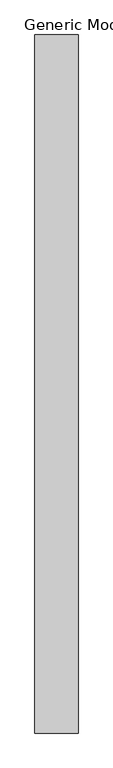
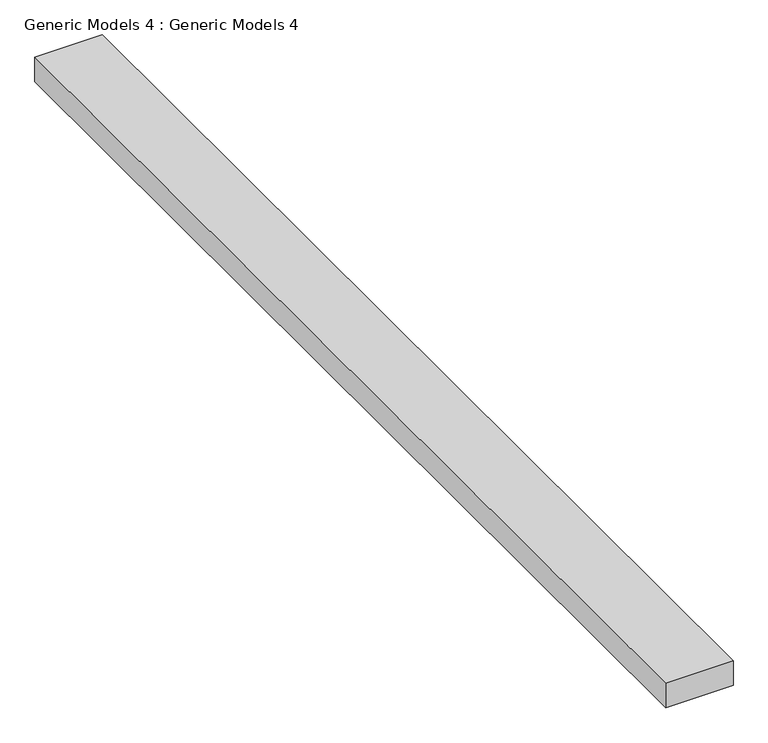
"""IFC4 building model written with IfcOpenShell, lengths in millimetres: proxy geometry, Generic Models 4 : Generic Models 4."""

from ifc_helpers import new_model, si_unit, frame, origin, place, context, project, spatial, polyline, outline, extrude, source, transform, mapped, element, save


def generic_models_4_generic_models_4_f29f5d5a(model_context):
    return source(origin(), model_context, "Body", "SweptSolid", [
        extrude(outline(polyline([(14902.7853663, -32.3497958), (14902.7853663, -12919.6493901), (14106.5361222, -12919.6493901), (14106.5361222, -32.3497958), (14902.7853663, -32.3497958)])), frame((0.0, 0.0, 6096.0), z_axis=(0.0, 0.0, 1.0), x_axis=(1.0, 0.0, 0.0)), (0.0, 0.0, 1.0), 304.8),
    ])


if __name__ == "__main__":
    model = new_model("IFC4")
    model_context = context("Model", 3, world=origin())
    ifc_project = project(units=[si_unit("LENGTHUNIT", "METRE", prefix="MILLI")], contexts=[model_context])
    site = spatial("IfcSite", under=ifc_project)
    building = spatial("IfcBuilding", under=site)
    placement = place(None, origin())
    generic_models_4_generic_models_4_shape = generic_models_4_generic_models_4_f29f5d5a(model_context)
    element("IfcBuildingElementProxy", 1, Name="Generic Models 4 : Generic Models 4", ObjectType="Generic Models 4 : Generic Models 4", at=placement, inside=building, context=model_context, shape_type="MappedRepresentation", body=[
        mapped(generic_models_4_generic_models_4_shape, transform((0.0, 0.0, 0.0), x_axis=(1.0, 0.0, 0.0), y_axis=(0.0, 1.0, 0.0), z_axis=(0.0, 0.0, 1.0))),
    ])
    save(model, "model.ifc")
